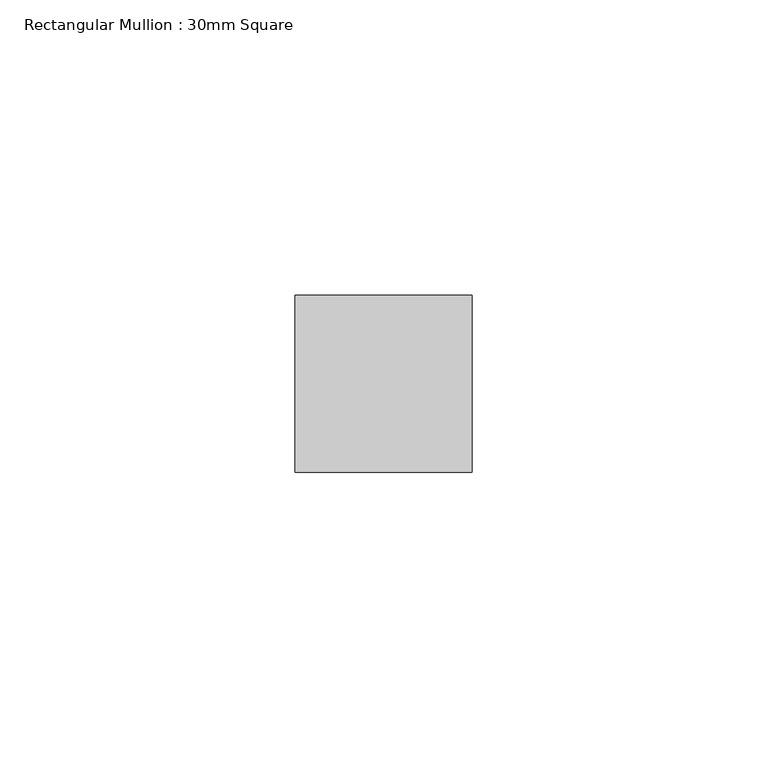
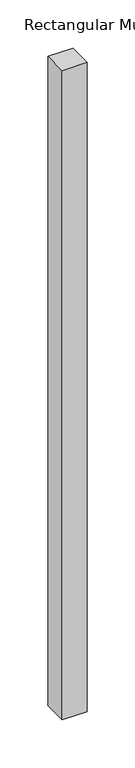
"""IFC4 building model written with IfcOpenShell, lengths in millimetres: member geometry, Rectangular Mullion : 30mm Square."""

from ifc_helpers import new_model, si_unit, frame, origin, place, context, project, spatial, polyline, outline, extrude, source, transform, mapped, element, save


def rectangular_mullion_30mm_square_741b6552(model_context):
    return source(origin(), model_context, "Body", "SweptSolid", [
        extrude(outline(polyline([(0.0, 15.0), (0.0, -15.0), (-30.0, -15.0), (-30.0, 15.0), (0.0, 15.0)])), frame((0.0, 0.0, -825.0), z_axis=(0.0, 0.0, 1.0), x_axis=(1.0, 0.0, 0.0)), (0.0, 0.0, 1.0), 825.0),
    ])


if __name__ == "__main__":
    model = new_model("IFC4")
    model_context = context("Model", 3, world=origin())
    ifc_project = project(units=[si_unit("LENGTHUNIT", "METRE", prefix="MILLI")], contexts=[model_context])
    site = spatial("IfcSite", under=ifc_project)
    building = spatial("IfcBuilding", under=site)
    placement = place(None, origin())
    rectangular_mullion_30mm_square_shape = rectangular_mullion_30mm_square_741b6552(model_context)
    element("IfcMember", 1, ObjectType="Rectangular Mullion : 30mm Square", at=placement, inside=building, context=model_context, shape_type="MappedRepresentation", body=[
        mapped(rectangular_mullion_30mm_square_shape, transform((0.0, 0.0, 0.0), x_axis=(1.0, 0.0, 0.0), y_axis=(0.0, 1.0, 0.0), z_axis=(0.0, 0.0, 1.0))),
    ])
    save(model, "model.ifc")

# Revit data of these elements
# Type "Rectangular Mullion : 30mm Square"
#   built-in parameter 1007304 = 0.0984252 (stored number, unit not read)
#   built-in parameter 1007301 = 0.0492126 (stored number, unit not read)
#   built-in parameter 1007300 = 0.0492126 (stored number, unit not read)
# Element 1 (IfcMember, "Rectangular Mullion : 30mm Square")
#   Materials on its faces: "Aluminum"
# Materials
#   "Aluminum": class "Metal", colour RGB 244 244 244, transparency 0, Description = "Aluminum 6061", Cost = 0
